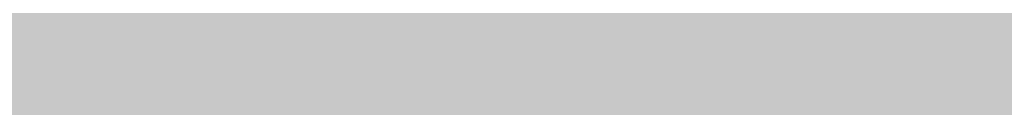
# Model space of a CAD drawing. Units: inches. Extents: x 2091 to 2899, y 967 to 2217.
# Tile 201 of 256: x 2203.18039 to 2203.25707, y 1152.25378 to 1152.26051. Entities that reach past the tile are written whole.
import ezdxf

# ---------------------------------------------------------------- set-up
doc = ezdxf.new("R2010")
doc.units = ezdxf.units.IN
doc.layers.add('A-WALL-PATT', color=141, linetype='Continuous', lineweight=13, true_color=0xadddf7)

msp = doc.modelspace()

# ---------------------------------------------------------------- hatches: boundary and pattern name
at = {"layer": 'A-WALL-PATT'}
h = msp.add_hatch(color=256, dxfattribs=at)
h.dxf.hatch_style = 1
h.paths.add_polyline_path([(2803.143603, 2050.919059), (2203.143603, 2050.919059), (2203.143603, 1090.919059), (2803.143603, 1090.919059)])
h.paths.add_polyline_path([(2635.79885, 1147.540465), (2674.524052, 1147.540465, 0.376086), (2678.529665, 1152.880202), (2678.529665, 1159.556473, 0.333335), (2674.524319, 1163.561846), (2674.524319, 1163.56185), (2674.524319, 1192.93439), (2635.805971, 1192.93439), (2597.087622, 1192.93439), (2597.087622, 1163.561846, 0.333335), (2593.082276, 1159.556473), (2593.082276, 1152.880202, 0.376086), (2597.087889, 1147.540465)], flags=0)
h.paths.add_polyline_path([(2436.010433, 1278.240778, 0.000483), (2435.952643, 1278.215027, -0.001328), (2435.935625, 1278.111693, -0.001711), (2436.11644, 1278.040758, 0.002185)], flags=0)
h.paths.add_polyline_path([(2794.143603, 1143.419059), (2794.143603, 1347.419059), (2543.370171, 1347.419059), (2543.370171, 1351.919059), (2794.143603, 1351.919059), (2794.143603, 1392.713555), (2793.947398, 1392.713555), (2793.947398, 1473.5369), (2794.143603, 1473.5369), (2794.143603, 1531.919059), (2650.143603, 1531.919059), (2650.143603, 1536.419059), (2794.143603, 1536.419059), (2794.143603, 1692.419059), (2609.375609, 1692.419059), (2609.375609, 1644.419059), (2604.875609, 1644.419059), (2604.875609, 1744.919059), (2609.375609, 1744.919059), (2609.375609, 1696.919059), (2794.143603, 1696.919059), (2794.143603, 1780.919059), (2609.643603, 1780.919059), (2493.875609, 1780.919059), (2493.875609, 1785.419059), (2609.643603, 1785.419059), (2794.143603, 1785.419059), (2794.143603, 1847.938821), (2793.951222, 1847.938821), (2793.951222, 1928.762166), (2794.143603, 1928.762166), (2794.143603, 1941.419059), (2614.143603, 1941.419059), (2614.143603, 1821.419059), (2609.643603, 1821.419059), (2609.643603, 1941.419059), (2392.143603, 1941.419059), (2392.143603, 1819.919059), (2387.643603, 1819.919059), (2387.643603, 1941.419059), (2212.143603, 1941.419059), (2212.143603, 1783.919059), (2392.143603, 1783.919059), (2392.143603, 1780.919059), (2212.143603, 1780.919059), (2212.143603, 1629.419059), (2387.643603, 1629.419059), (2387.643603, 1744.919059), (2392.143603, 1744.919059), (2392.143603, 1627.919059), (2317.143603, 1627.919059), (2317.143603, 1551.419059), (2317.143603, 1536.419059), (2459.383591, 1536.419059), (2459.383591, 1602.39648), (2463.883591, 1602.39648), (2463.883591, 1531.919059), (2456.643603, 1531.919059), (2456.643603, 1529.919059), (2452.143603, 1529.919059), (2452.143603, 1531.919059), (2312.643603, 1531.919059), (2312.643603, 1551.419059), (2306.143603, 1551.419059), (2306.143603, 1555.919059), (2308.143603, 1555.919059), (2308.143603, 1551.419059), (2312.643603, 1551.419059), (2312.643603, 1627.919059), (2212.143603, 1627.919059), (2212.143603, 1555.919059), (2270.143603, 1555.919059), (2270.143603, 1551.419059), (2212.143603, 1551.419059), (2212.143603, 1351.919059), (2272.143603, 1351.919059), (2272.143603, 1347.419059), (2212.143603, 1347.419059), (2212.143603, 1275.419059), (2308.143603, 1275.419059), (2308.143603, 1351.919059), (2452.143603, 1351.919059), (2452.143603, 1493.919059), (2456.643603, 1493.919059), (2456.643603, 1347.419059), (2312.643603, 1347.419059), (2312.643603, 1270.919059), (2212.143603, 1270.919059), (2212.143603, 1099.919059), (2281.237523, 1099.919059), (2282.871041, 1110.913803), (2282.008341, 1116.996603), (2278.557741, 1121.420403), (2268.205641, 1128.056203), (2272.087641, 1128.056203), (2273.812941, 1131.927003), (2279.420341, 1134.691903), (2285.027841, 1135.244903), (2287.615841, 1137.456803), (2288.047141, 1138.009803), (2289.341141, 1140.774703), (2291.066541, 1139.668703), (2292.360541, 1135.244903), (2295.379841, 1136.903803), (2296.242541, 1135.797903), (2297.105241, 1133.033003), (2300.124641, 1138.009803), (2303.143941, 1138.009803), (2304.437941, 1135.797903), (2303.143941, 1133.586003), (2306.594641, 1134.691903), (2307.888741, 1133.033003), (2310.908041, 1135.244903), (2313.927441, 1134.138903), (2315.62686, 1132.427102), (2308.320041, 1117.549603), (2290.203841, 1109.807903), (2288.909841, 1103.172103), (2289.272309, 1099.919059), (2434.918227, 1099.919059), (2431.593227, 1124.788059), (2429.930227, 1169.553059), (2430.927185, 1240.519694), (2435.658926, 1238.186126), (2437.135227, 1196.554059), (2438.798227, 1143.973059), (2442.678227, 1111.998059), (2446.558227, 1099.919059), (2794.143603, 1099.919059), (2794.143603, 1138.919059), (2548.032447, 1138.919059), (2548.032447, 1143.419059), (2548.032447, 1148.819059), (2546.668457, 1148.031559), (2528.685692, 1179.178622, 0.256256), (2512.032447, 1148.819059), (2512.032447, 1143.419059), (2512.032447, 1138.919059), (2507.532447, 1138.919059), (2507.532447, 1143.419059), (2507.532447, 1148.819059, 0.256256), (2490.879202, 1179.178622), (2472.896437, 1148.031559), (2471.532447, 1148.819059), (2471.532447, 1143.419059), (2467.032447, 1143.419059), (2467.032447, 1269.945786, 0.039061), (2460.909987, 1273.580059), (2467.032447, 1273.580059), (2467.032447, 1286.325364, 0.014511), (2465.216194, 1286.761905), (2467.032447, 1287.052576), (2467.032447, 1323.419059), (2471.532447, 1323.419059), (2471.532447, 1148.819059), (2489.532447, 1179.995973), (2490.896437, 1179.208473), (2490.879202, 1179.178622, -0.256256), (2507.532447, 1148.819059), (2507.532447, 1143.419059), (2512.032447, 1143.419059), (2512.032447, 1148.819059, -0.256256), (2528.685692, 1179.178622), (2528.668457, 1179.208473), (2530.032447, 1179.995973), (2548.032447, 1148.819059), (2548.032447, 1143.419059)], flags=16)
h.paths.add_polyline_path([(2607.768546, 1200.945083), (2607.768546, 1265.030625), (2597.087622, 1281.052011), (2619.784585, 1281.052011), (2627.795278, 1337.12686), (2635.79885, 1337.12686), (2643.816663, 1337.12686), (2651.827356, 1281.052011), (2674.524319, 1281.052011), (2663.843395, 1265.030625), (2663.843395, 1200.945083), (2635.805971, 1200.945083)], flags=0)
edge = h.paths.add_edge_path(flags=0)
edge.add_ellipse((13303.896215, 1272.998725), major_axis=(-10595.31304, 0.000001), ratio=0.842303870086, start_angle=0.6282372191, end_angle=0.6465540999, ccw=False)
edge.add_ellipse((2711.70045, 1156.852678), major_axis=(2.219769, 0), ratio=0.84230387, start_angle=111.535244, end_angle=180.628237, ccw=False)
edge.add_ellipse((13303.156292, 1272.998725), major_axis=(-10593.026306, 0), ratio=0.842303869544, start_angle=0.5282714718, end_angle=0.6465540971, ccw=False)
edge.add_line((2710.764596, 1175.333295), (2710.129986, 1175.333295))
edge.add_ellipse((2710.129986, 1176.579775), major_axis=(1.479846, 0), ratio=0.84230387, start_angle=180, end_angle=270, ccw=False)
edge.add_line((2708.65014, 1176.579775), (2708.65014, 1200.782914))
edge.add_ellipse((2710.129986, 1200.782914), major_axis=(1.479846, 0), ratio=0.84230387, start_angle=90, end_angle=180, ccw=False)
edge.add_line((2710.129986, 1202.029394), (2710.465075, 1202.029394))
edge.add_ellipse((13303.156292, 1272.998725), major_axis=(-10593.026306, 0), ratio=0.842303869544, start_angle=-0.0902290886, end_angle=0.3838667788, ccw=False)
edge.add_ellipse((2710.129986, 1290.927031), major_axis=(-1.479846, 0), ratio=0.84230387, start_angle=0, end_angle=90, ccw=False)
edge.add_line((2708.65014, 1290.927031), (2708.65014, 1315.13017))
edge.add_ellipse((2710.129986, 1315.13017), major_axis=(-1.479846, 0), ratio=0.84230387, start_angle=-90, end_angle=0, ccw=False)
edge.add_line((2710.129986, 1316.37665), (2710.706314, 1316.37665))
edge.add_ellipse((3238.40172, 1296.289566), major_axis=(528.234, 0), ratio=0.8423038695, start_angle=176.34957241, end_angle=177.82004969, ccw=False)
edge.add_ellipse((2775.063043, 1071.450696), major_axis=(313.307761, 0), ratio=0.8423038695, start_angle=102.12596555, end_angle=103.78052899, ccw=False)
edge.add_ellipse((2775.063043, 1078.305698), major_axis=(-305.302891, 0), ratio=0.8423038695, start_angle=-79.790461, end_angle=-77.55537271, ccw=False)
edge.add_ellipse((2695.141767, 1541.975383), major_axis=(-250.960216, 0), ratio=0.8423038695, start_angle=99.25656601, end_angle=102.55493264)
edge.add_line((2741.410326, 1334.214255), (2747.132545, 1337.378477))
edge.add_ellipse((2747.538616, 1336.857478), major_axis=(-0.739923, 0), ratio=0.8423039, start_angle=270, end_angle=307.93313, ccw=False)
edge.add_ellipse((2747.538616, 1336.857478), major_axis=(-0.739923, 0), ratio=0.8423039, start_angle=232.06687, end_angle=270, ccw=False)
edge.add_line((2747.944687, 1337.378477), (2753.666906, 1334.214255))
edge.add_ellipse((2799.935466, 1541.975383), major_axis=(250.960216, 0), ratio=0.8423038695, start_angle=257.44506736, end_angle=260.74343399)
edge.add_ellipse((2720.014189, 1078.305698), major_axis=(305.302891, 0), ratio=0.8423038695, start_angle=77.55537271, end_angle=79.790461, ccw=False)
edge.add_ellipse((2720.014189, 1071.450696), major_axis=(-313.307761, 0), ratio=0.8423038695, start_angle=256.21947101, end_angle=257.87403445, ccw=False)
edge.add_ellipse((2256.675512, 1296.289566), major_axis=(-528.234, 0), ratio=0.8423038695, start_angle=182.17995031, end_angle=183.65042759, ccw=False)
edge.add_line((2784.370918, 1316.37665), (2784.947247, 1316.37665))
edge.add_ellipse((2784.947247, 1315.13017), major_axis=(1.479846, 0), ratio=0.84230387, start_angle=0, end_angle=90, ccw=False)
edge.add_line((2786.427093, 1315.13017), (2786.427093, 1290.927031))
edge.add_ellipse((2784.947247, 1290.927031), major_axis=(1.479846, 0), ratio=0.84230387, start_angle=270, end_angle=360, ccw=False)
edge.add_ellipse((-7808.07906, 1272.998725), major_axis=(10593.026306, 0), ratio=0.842303869544, start_angle=-0.3838667788, end_angle=0.0902290886, ccw=False)
edge.add_line((2784.612157, 1202.029394), (2784.947247, 1202.029394))
edge.add_ellipse((2784.947247, 1200.782914), major_axis=(1.479846, 0), ratio=0.84230387, start_angle=0, end_angle=90, ccw=False)
edge.add_line((2786.427093, 1200.782914), (2786.427093, 1176.579775))
edge.add_ellipse((2784.947247, 1176.579775), major_axis=(-1.479846, 0), ratio=0.84230387, start_angle=90, end_angle=180, ccw=False)
edge.add_line((2784.947247, 1175.333295), (2784.312636, 1175.333295))
edge.add_ellipse((-7808.07906, 1272.998725), major_axis=(10593.026306, 0), ratio=0.842303869544, start_angle=-0.6186431963, end_angle=-0.5282714718, ccw=False)
edge.add_ellipse((2783.376783, 1156.852678), major_axis=(-2.219769, 0), ratio=0.84230387, start_angle=179.371763, end_angle=248.464757, ccw=False)
edge.add_ellipse((-7808.818983, 1272.998725), major_axis=(-10595.31304, 0.000004), ratio=0.842303865762, start_angle=179.3534459226, end_angle=179.3717628034, ccw=False)
edge.add_ellipse((2780.297303, 1153.500793), major_axis=(-5.246426, 0), ratio=0.84230387, start_angle=90, end_angle=179.353446, ccw=False)
edge.add_line((2780.297303, 1149.081708), (2714.77993, 1149.081708))
edge.add_ellipse((2714.77993, 1153.500793), major_axis=(5.246426, 0), ratio=0.84230387, start_angle=180.646554, end_angle=270, ccw=False)
edge = h.paths.add_edge_path(flags=0)
edge.add_line((2718.187367, 1151.007833), (2718.187367, 1170.472364))
edge.add_ellipse((2721.14706, 1170.472364), major_axis=(-2.959692, 0), ratio=0.84230387, start_angle=-90, end_angle=0, ccw=False)
edge.add_line((2721.14706, 1172.965324), (2773.930173, 1172.965324))
edge.add_ellipse((2773.930173, 1170.472364), major_axis=(-2.959692, 0), ratio=0.84230387, start_angle=180, end_angle=270, ccw=False)
edge.add_line((2776.889865, 1170.472364), (2776.889865, 1151.007833))
edge.add_line((2776.889865, 1151.007833), (2718.187367, 1151.007833))
edge = h.paths.add_edge_path(flags=0)
edge.add_line((2718.187367, 1180.23415), (2718.187367, 1199.057834))
edge.add_ellipse((2747.538616, 1320.39864), major_axis=(147.017924, 0), ratio=0.8423038695, start_angle=256.40186531, end_angle=283.59813469)
edge.add_line((2776.889865, 1199.057834), (2776.889865, 1180.23415))
edge.add_ellipse((2747.538616, 1301.574956), major_axis=(147.017924, 0), ratio=0.8423038695, start_angle=256.40186531, end_angle=283.59813469, ccw=False)
edge = h.paths.add_edge_path(flags=0)
edge.add_ellipse((13303.156292, 1272.998725), major_axis=(-10591.54646, 0), ratio=0.842303869555, start_angle=0.0555943135, end_angle=0.3777641939, ccw=False)
edge.add_line((2711.616859, 1262.72171), (2715.667408, 1249.495396))
edge.add_ellipse((6413.891963, 1241.691919), major_axis=(-3698.236159, 0), ratio=0.84230386955, start_angle=-0.120897369, end_angle=0.364076349)
edge.add_line((2715.761038, 1218.192455), (2711.934307, 1203.167361))
edge = h.paths.add_edge_path(flags=0)
edge.add_line((2718.187367, 1251.074566), (2716.002485, 1267.450435))
edge.add_ellipse((2742.151175, 1202.18954), major_axis=(81.772585, 0), ratio=0.84230387, start_angle=94.27742096, end_angle=111.8349538, ccw=False)
edge.add_line((2737.009748, 1270.930626), (2758.067484, 1270.930626))
edge.add_ellipse((2752.926058, 1202.18954), major_axis=(81.772585, 0), ratio=0.84230387, start_angle=68.1650462, end_angle=85.72257904, ccw=False)
edge.add_line((2779.074747, 1267.450435), (2776.889865, 1251.074566))
edge.add_ellipse((2750.338059, 1187.885356), major_axis=(79.579664, 0), ratio=0.84230387, start_angle=67.20808512, end_angle=85.1299304)
edge.add_line((2756.034656, 1254.743656), (2739.042576, 1254.743656))
edge.add_ellipse((2744.739174, 1187.885356), major_axis=(79.579664, 0), ratio=0.84230387, start_angle=94.8700696, end_angle=112.79191488)
edge = h.paths.add_edge_path(flags=0)
edge.add_line((2783.142926, 1203.167361), (2779.316194, 1218.192455))
edge.add_ellipse((-918.81473, 1241.691919), major_axis=(3698.236159, 0), ratio=0.84230386955, start_angle=-0.364076349, end_angle=0.120897369)
edge.add_line((2779.409825, 1249.495396), (2783.460373, 1262.72171))
edge.add_ellipse((-7808.07906, 1272.998725), major_axis=(-10591.54646, 0), ratio=0.84230386954, start_angle=179.6222358061, end_angle=179.9444056865, ccw=False)
edge = h.paths.add_edge_path(flags=0)
edge.add_ellipse((2734.200892, 1286.69044), major_axis=(-0.356609, 6.340078), ratio=0.60383358, start_angle=89.0020143, end_angle=253.657408, ccw=False)
edge.add_line((2730.369001, 1286.541806), (2730.369001, 1301.35198))
edge.add_line((2730.369001, 1301.35198), (2735.913311, 1305.214803))
edge.add_ellipse((2736.384917, 1304.734561), major_axis=(0.739923, 0), ratio=0.8423039, start_angle=90, end_angle=134.480211, ccw=False)
edge.add_line((2736.384917, 1305.357801), (2738.032783, 1305.357801))
edge.add_line((2738.032783, 1305.357801), (2738.032783, 1307.707927))
edge.add_ellipse((2794.201642, 1307.707927), major_axis=(56.168859, 0), ratio=0.84230387, start_angle=150.5614304, end_angle=180, ccw=False)
edge.add_ellipse((2700.875591, 1307.707927), major_axis=(-56.168859, 0), ratio=0.84230387, start_angle=180, end_angle=209.4385696, ccw=False)
edge.add_line((2757.04445, 1307.707927), (2757.04445, 1305.357801))
edge.add_line((2757.04445, 1305.357801), (2758.692316, 1305.357801))
edge.add_ellipse((2758.692316, 1304.734561), major_axis=(-0.739923, 0), ratio=0.8423039, start_angle=225.519789, end_angle=270, ccw=False)
edge.add_line((2759.163922, 1305.214803), (2764.708231, 1301.35198))
edge.add_line((2764.708231, 1301.35198), (2764.708231, 1286.541806))
edge.add_ellipse((2760.87634, 1286.69044), major_axis=(0.356609, 6.340078), ratio=0.60383358, start_angle=106.342592, end_angle=270.9979857, ccw=False)
edge.add_line((2757.04445, 1285.79709), (2757.04445, 1307.707927))
edge.add_ellipse((2700.875591, 1307.707927), major_axis=(-56.168859, 0), ratio=0.84230387, start_angle=180, end_angle=209.4385696)
edge.add_ellipse((2794.201642, 1307.707927), major_axis=(56.168859, 0), ratio=0.84230387, start_angle=150.5614304, end_angle=180)
edge.add_line((2738.032783, 1307.707927), (2738.032783, 1285.79709))
h.paths.add_polyline_path([(2417.812273, 1104.449704), (2413.492273, 1102.529704), (2410.612273, 1103.969704), (2409.172273, 1106.369704), (2407.252273, 1107.329704), (2406.292273, 1109.729704), (2405.332273, 1114.049704), (2405.332273, 1117.889704), (2406.292273, 1120.129704), (2407.252273, 1119.809704), (2408.848322, 1118.327658), (2410.173945, 1119.42417), (2410.211273, 1120.405704), (2411.040731, 1121.419054), (2410.699273, 1119.858704), (2410.173945, 1119.42417), (2410.088452, 1117.176109), (2411.132836, 1116.206324), (2413.972273, 1119.329704), (2416.852273, 1120.769704), (2416.869721, 1120.798784), (2417.035071, 1119.405116), (2417.896213, 1118.143384), (2418.292273, 1118.369704), (2419.544447, 1120.039269), (2419.360915, 1118.387487), (2419.032108, 1119.356151), (2418.398939, 1118.511926), (2419.252273, 1114.529704), (2418.794091, 1107.198795)], flags=0)
h.paths.add_polyline_path([(2508.870171, 1347.419059), (2508.370171, 1347.419059), (2508.370171, 1351.919059), (2508.870171, 1351.919059)], flags=0)
h.paths.add_polyline_path([(2473.370171, 1347.419059), (2472.370171, 1347.419059), (2467.870171, 1347.419059), (2467.870171, 1455.419059), (2472.370171, 1455.419059), (2472.370171, 1352.419059), (2473.370171, 1352.419059)], flags=0)
h.paths.add_polyline_path([(2352.106244, 1217.446197), (2349.226244, 1218.886197), (2347.786244, 1221.286197), (2345.866244, 1222.246197), (2344.906244, 1224.646197), (2343.946244, 1228.966197), (2343.946244, 1232.806197), (2344.906244, 1235.046197), (2345.866244, 1234.726197), (2347.462293, 1233.244152), (2348.787916, 1234.340663), (2348.825244, 1235.322197), (2349.654702, 1236.335547), (2349.313244, 1234.775197), (2348.787916, 1234.340663), (2348.702423, 1232.092603), (2349.746807, 1231.122817), (2352.586244, 1234.246197), (2355.466244, 1235.686197), (2355.483692, 1235.715277), (2355.649043, 1234.321609), (2356.510185, 1233.059877), (2356.906244, 1233.286197), (2358.158418, 1234.955762), (2357.974887, 1233.30398), (2357.646079, 1234.272644), (2357.012911, 1233.428419), (2357.866244, 1229.446197), (2357.408062, 1222.115288), (2356.426244, 1219.366197)], flags=0)
h.paths.add_polyline_path([(2348.2968, 1112.22442), (2347.0138, 1112.31042), (2345.5298, 1114.12742), (2345.7318, 1115.85842), (2346.8118, 1116.98242), (2346.8118, 1114.64642), (2345.8668, 1114.21442), (2346.8798, 1114.30042)], flags=0)
h.paths.add_polyline_path([(2347.0138, 1110.92642), (2346.2718, 1110.49342), (2346.6098, 1111.18642)], flags=0)
h.paths.add_polyline_path([(2345.8668, 1118.19442), (2345.5298, 1117.32942), (2343.7078, 1118.02142), (2344.3828, 1118.62642)], flags=0)
h.paths.add_polyline_path([(2346.6768, 1109.28242), (2346.0698, 1108.07142), (2345.8668, 1110.06142)], flags=0)
h.paths.add_polyline_path([(2345.0568, 1119.75142), (2343.6398, 1119.75142), (2343.9778, 1121.13542)], flags=0)
h.paths.add_polyline_path([(2345.2598, 1116.55042), (2345.1248, 1115.85842), (2344.9218, 1115.68542), (2344.7198, 1116.37742)], flags=0)
h.paths.add_polyline_path([(2345.6648, 1112.31042), (2345.4618, 1111.53242), (2344.0448, 1111.96442), (2344.6518, 1112.57042)], flags=0)
h.paths.add_polyline_path([(2345.1918, 1113.34942), (2344.4498, 1113.86842), (2344.7198, 1114.38742)], flags=0)
h.paths.add_polyline_path([(2344.6518, 1116.80942), (2344.1798, 1115.68542), (2344.6518, 1115.33942), (2343.9098, 1114.90642), (2343.0328, 1115.94442), (2343.6398, 1116.46342)], flags=0)
h.paths.add_polyline_path([(2345.8668, 1106.68642), (2344.9898, 1105.56242), (2344.5168, 1106.60042)], flags=0)
h.paths.add_polyline_path([(2344.8548, 1110.06142), (2344.5168, 1109.28242), (2344.1128, 1109.71542)], flags=0)
h.paths.add_polyline_path([(2344.0448, 1113.52242), (2343.4378, 1113.08942), (2342.7628, 1113.95442)], flags=0)
h.paths.add_polyline_path([(2344.3148, 1111.01242), (2342.9648, 1110.32042), (2342.9648, 1111.09942)], flags=0)
h.paths.add_polyline_path([(2345.1248, 1104.69742), (2344.5848, 1103.74542), (2344.4498, 1104.26442)], flags=0)
h.paths.add_polyline_path([(2342.8298, 1121.22242), (2341.7498, 1120.53042), (2340.5358, 1121.04942), (2340.1308, 1121.82842), (2340.6708, 1122.95242), (2341.1428, 1121.82842), (2341.6148, 1122.00142)], flags=0)
h.paths.add_polyline_path([(2342.9648, 1119.75142), (2343.0328, 1118.45342), (2342.0878, 1118.02142), (2342.0198, 1119.49142)], flags=0)
h.paths.add_polyline_path([(2342.6948, 1116.89642), (2341.9528, 1116.63642), (2342.0198, 1117.32942)], flags=0)
h.paths.add_polyline_path([(2343.0328, 1112.22442), (2342.0198, 1111.79142), (2341.5478, 1112.22442), (2342.3578, 1113.34942)], flags=0)
h.paths.add_polyline_path([(2343.7748, 1104.43742), (2342.6278, 1102.88042), (2342.6948, 1104.61042), (2343.4378, 1105.12942)], flags=0)
h.paths.add_polyline_path([(2342.0198, 1115.07942), (2340.8058, 1115.51242), (2340.9408, 1116.37742)], flags=0)
h.paths.add_polyline_path([(2341.4808, 1120.09742), (2341.4808, 1119.40542), (2341.0758, 1119.57842), (2341.1428, 1120.09742)], flags=0)
h.paths.add_polyline_path([(2341.8178, 1114.47342), (2340.9408, 1113.08942), (2340.8058, 1114.56042)], flags=0)
h.paths.add_polyline_path([(2341.1428, 1118.54042), (2340.9408, 1116.98242), (2339.0508, 1117.67542), (2339.0508, 1118.62642)], flags=0)
h.paths.add_polyline_path([(2342.6948, 1101.66842), (2341.9528, 1101.84142), (2342.5598, 1102.36142)], flags=0)
h.paths.add_polyline_path([(2340.3328, 1119.66542), (2338.4438, 1119.57842), (2337.9038, 1120.35742), (2339.6578, 1120.61642)], flags=0)
h.paths.add_polyline_path([(2340.3328, 1115.33942), (2340.0628, 1113.69542), (2339.3878, 1115.33942)], flags=0)
h.paths.add_polyline_path([(2341.8178, 1103.83142), (2341.5478, 1102.88042), (2341.1428, 1103.65842)], flags=0)
h.paths.add_polyline_path([(2339.0508, 1122.86642), (2337.2958, 1121.82842), (2337.0938, 1123.12542), (2337.7688, 1123.81842)], flags=0)
h.paths.add_polyline_path([(2339.1178, 1121.74142), (2338.8478, 1121.22242), (2338.1738, 1121.04942), (2338.3758, 1121.56842)], flags=0)
h.paths.add_polyline_path([(2339.1858, 1119.31942), (2338.6458, 1118.71342), (2338.2408, 1118.10742), (2338.2408, 1118.88642)], flags=0)
h.paths.add_polyline_path([(2341.1428, 1101.92842), (2340.6028, 1101.23642), (2340.0628, 1101.84142), (2340.6028, 1102.36142)], flags=0)
h.paths.add_polyline_path([(2337.6338, 1117.76142), (2336.6208, 1118.28042), (2337.2958, 1118.97242)], flags=0)
h.paths.add_polyline_path([(2336.8238, 1119.57842), (2334.7988, 1118.97242), (2335.2038, 1120.35742), (2336.5538, 1120.87642)], flags=0)
h.paths.add_polyline_path([(2339.1178, 1100.45742), (2337.3638, 1100.54342), (2336.7558, 1101.23642)], flags=0)
h.paths.add_polyline_path([(2336.3508, 1122.43342), (2336.0138, 1121.91442), (2334.9338, 1122.43342), (2334.5288, 1123.47142), (2335.7438, 1122.77942)], flags=0)
h.paths.add_polyline_path([(2334.7318, 1120.87642), (2334.2588, 1120.35742), (2334.0568, 1120.78942), (2334.5968, 1121.30842)], flags=0)
h.paths.add_polyline_path([(2334.4618, 1122.17442), (2332.5718, 1121.30842), (2331.3568, 1122.17442), (2332.0998, 1122.86642)], flags=0)
h.paths.add_polyline_path([(2334.2588, 1118.54042), (2333.3818, 1118.45342), (2333.6518, 1119.31942)], flags=0)
h.paths.add_polyline_path([(2335.5418, 1102.27442), (2334.1918, 1102.62042), (2335.2718, 1103.31242)], flags=0)
h.paths.add_polyline_path([(2332.7068, 1119.66542), (2331.6948, 1120.44342), (2332.5048, 1120.78942)], flags=0)
h.paths.add_polyline_path([(2334.7318, 1101.14942), (2333.5168, 1101.58242), (2333.9888, 1101.75542)], flags=0)
h.paths.add_polyline_path([(2332.6398, 1116.63642), (2331.0868, 1116.29042), (2331.9648, 1118.19442)], flags=0)
h.paths.add_polyline_path([(2330.7498, 1121.56842), (2330.2768, 1120.27042), (2328.5228, 1119.31942), (2328.9948, 1121.04942)], flags=0)
h.paths.add_polyline_path([(2330.7498, 1118.62642), (2330.0078, 1117.50242), (2329.8728, 1118.02142)], flags=0)
h.paths.add_polyline_path([(2332.0998, 1102.36142), (2330.5468, 1102.01442), (2331.6948, 1102.96642)], flags=0)
h.paths.add_polyline_path([(2329.5348, 1113.60842), (2329.0628, 1112.31042), (2328.5898, 1113.34942)], flags=0)
h.paths.add_polyline_path([(2328.3878, 1117.84842), (2327.5098, 1116.55042), (2327.1728, 1117.76142)], flags=0)
h.paths.add_polyline_path([(2329.7378, 1106.51342), (2329.5348, 1105.30242), (2328.2528, 1106.08142)], flags=0)
h.paths.add_polyline_path([(2328.6578, 1114.38742), (2328.0498, 1114.12742), (2328.3198, 1114.90642)], flags=0)
h.paths.add_polyline_path([(2328.3198, 1112.22442), (2327.1058, 1112.13742), (2326.7008, 1112.65642)], flags=0)
h.paths.add_polyline_path([(2326.9028, 1115.25242), (2326.7008, 1114.12742), (2325.2158, 1113.60842), (2326.0928, 1115.33942)], flags=0)
h.paths.add_polyline_path([(2326.6328, 1108.33042), (2326.0928, 1107.37942), (2325.8908, 1108.50342), (2326.4978, 1109.10942)], flags=0)
h.paths.add_polyline_path([(2615.143603, 1531.919059), (2609.643603, 1531.919059), (2609.643603, 1620.419059), (2614.143603, 1620.419059), (2614.143603, 1536.419059), (2615.143603, 1536.419059)], flags=0)
h.paths.add_polyline_path([(2545.143603, 1563.419059), (2464.143603, 1563.419059), (2464.143603, 1632.419059), (2509.143603, 1632.419059), (2509.143603, 1627.919059), (2509.143603, 1603.919059), (2468.643603, 1603.919059), (2468.643603, 1567.919059), (2540.643603, 1567.919059), (2540.643603, 1591.919059), (2545.143603, 1591.919059)], flags=0)
h.paths.add_polyline_path([(2388.969048, 1549.985735), (2357.434181, 1549.985735), (2357.434181, 1623.360778), (2399.362777, 1623.360778), (2435.689465, 1623.360778), (2435.592547, 1602.559273), (2435.592547, 1602.39648), (2388.969048, 1602.39648)], flags=0)
h.paths.add_polyline_path([(2388.880628, 1555.809151), (2374.904429, 1555.809151), (2374.904429, 1600.571564), (2374.904429, 1615.457645), (2406.350877, 1615.457645), (2406.350877, 1618.939431), (2412.174293, 1615.457645), (2406.350877, 1611.97586), (2406.350877, 1615.457645), (2388.880628, 1615.457645)], flags=0)
h.paths.add_polyline_path([(2568.875609, 1644.419059), (2453.375609, 1644.419059), (2453.375609, 1785.419059), (2457.875609, 1785.419059), (2457.875609, 1648.919059), (2568.875609, 1648.919059)], flags=0)
h.paths.add_polyline_path([(2212.143603, 1945.919059), (2212.143603, 2041.919059), (2794.143603, 2041.919059), (2794.143603, 1945.919059)], flags=16)
h.paths.add_polyline_path([(2271.082728, 1964.317238), (2776.852968, 1964.317238), (2776.852968, 2037.169623), (2271.082728, 2037.169623)], flags=8)
h.paths.add_polyline_path([(2380.649285, 1536.824144), (2461.040809, 1536.824144), (2461.040809, 1554.652587), (2380.649285, 1554.652587)], flags=8)
h.paths.add_polyline_path([(2240.755709, 1609.725451), (2309.185829, 1609.725451), (2309.185829, 1617.698204), (2240.755709, 1617.698204)], flags=8)
h.paths.add_polyline_path([(2212.677255, 1313.504102), (2282.59152, 1313.504102), (2282.59152, 1322.745239), (2212.677255, 1322.745239)], flags=8)
h.paths.add_polyline_path([(2457.111976, 1114.778574), (2558.481581, 1114.778574), (2558.481581, 1142.219682), (2457.111976, 1142.219682)], flags=8)
h.paths.add_polyline_path([(2473.442337, 1273.010067), (2604.641226, 1273.010067), (2604.641226, 1318.346935), (2473.442337, 1318.346935)], flags=8)
h.paths.add_polyline_path([(2638.876302, 1626.977432), (2684.250367, 1627.976738), (2684.038483, 1637.597494), (2638.664417, 1636.598188)], flags=8)
h.paths.add_polyline_path([(2537.590554, 1453.793447), (2628.389547, 1453.793447), (2628.389547, 1475.344811), (2537.590554, 1475.344811)], flags=8)
h.paths.add_polyline_path([(2504.137638, 1714.632397), (2554.647187, 1714.632397), (2554.647187, 1730.237712), (2504.137638, 1730.237712)], flags=8)
h.paths.add_polyline_path([(2487.501181, 1575.651872), (2535.097121, 1575.651872), (2535.097121, 1598.377646), (2487.501181, 1598.377646)], flags=8)
h.paths.add_polyline_path([(2709.0994, 1735.710278), (2740.016601, 1735.710278), (2740.016601, 1749.937641), (2709.0994, 1749.937641)], flags=8)
h.paths.add_polyline_path([(2442.438424, 1792.171657), (2564.728835, 1792.171657), (2564.728835, 1842.000163), (2442.438424, 1842.000163)], flags=8)
h.paths.add_polyline_path([(2655.815801, 1809.644076), (2789.520142, 1806.693796), (2790.084977, 1832.291638), (2656.380635, 1835.241918)], flags=8)
h.paths.add_polyline_path([(2234.842697, 1797.720143), (2368.592851, 1794.768852), (2369.160718, 1820.504132), (2235.410564, 1823.455423)], flags=8)
h.paths.add_polyline_path([(2245.138466, 1644.006335), (2398.427733, 1640.6239), (2398.994842, 1666.32482), (2245.705575, 1669.707255)], flags=8)
h.paths.add_polyline_path([(2306.142847, 1431.168519), (2413.768314, 1428.793687), (2414.333148, 1454.391529), (2306.707682, 1456.76636)], flags=8)
h.paths.add_polyline_path([(2306.834582, 1458.233145), (2393.380484, 1456.323449), (2393.932808, 1481.354358), (2307.386907, 1483.264054)], flags=8)

doc.saveas('drawing.dxf')
